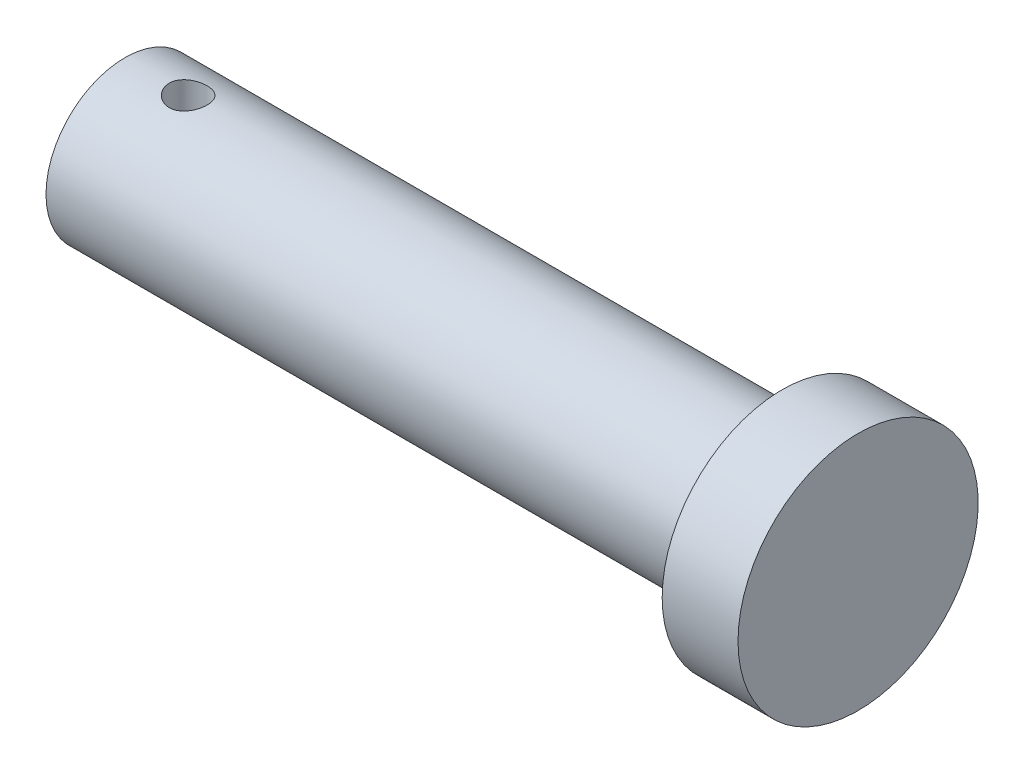
ISO-10303-21;
HEADER;
FILE_DESCRIPTION(('STEP AP214'),'2;1');
FILE_NAME('part.step','',(''),(''),'','','');
FILE_SCHEMA(('AUTOMOTIVE_DESIGN { 1 0 10303 214 1 1 1 1 }'));
ENDSEC;
DATA;
#1=APPLICATION_CONTEXT('core data for automotive mechanical design processes');
#2=APPLICATION_PROTOCOL_DEFINITION('international standard','automotive_design',2000,#1);
#3=PRODUCT_CONTEXT('',#1,'mechanical');
#4=PRODUCT('Part','Part','',(#3));
#5=PRODUCT_RELATED_PRODUCT_CATEGORY('part','',(#4));
#6=PRODUCT_DEFINITION_FORMATION('','',#4);
#7=PRODUCT_DEFINITION_CONTEXT('part definition',#1,'design');
#8=PRODUCT_DEFINITION('design','',#6,#7);
#9=PRODUCT_DEFINITION_SHAPE('','',#8);
#10=(LENGTH_UNIT() NAMED_UNIT(*) SI_UNIT(.MILLI.,.METRE.));
#11=(NAMED_UNIT(*) PLANE_ANGLE_UNIT() SI_UNIT($,.RADIAN.));
#12=(NAMED_UNIT(*) SI_UNIT($,.STERADIAN.) SOLID_ANGLE_UNIT());
#13=UNCERTAINTY_MEASURE_WITH_UNIT(LENGTH_MEASURE(1.E-05),#10,'distance_accuracy_value','');
#14=(GEOMETRIC_REPRESENTATION_CONTEXT(3) GLOBAL_UNCERTAINTY_ASSIGNED_CONTEXT((#13)) GLOBAL_UNIT_ASSIGNED_CONTEXT((#10,
#11,#12)) REPRESENTATION_CONTEXT('',''));
#15=CARTESIAN_POINT('',(0.,0.,0.));
#16=DIRECTION('',(0.,0.,1.));
#17=DIRECTION('',(1.,0.,0.));
#18=AXIS2_PLACEMENT_3D('',#15,#16,#17);
#19=CARTESIAN_POINT('',(0.,0.,0.));
#20=DIRECTION('',(-1.,0.,0.));
#21=DIRECTION('',(0.,0.,1.));
#22=AXIS2_PLACEMENT_3D('',#19,#20,#21);
#23=PLANE('',#22);
#24=CARTESIAN_POINT('',(0.,0.,0.));
#25=DIRECTION('',(-1.,0.,0.));
#26=DIRECTION('',(0.,0.,1.));
#27=AXIS2_PLACEMENT_3D('',#24,#25,#26);
#28=CIRCLE('',#27,12.5);
#29=CARTESIAN_POINT('',(0.,0.,12.5));
#30=VERTEX_POINT('',#29);
#31=EDGE_CURVE('E10',#30,#30,#28,.T.);
#32=ORIENTED_EDGE('',*,*,#31,.T.);
#33=EDGE_LOOP('',(#32));
#34=FACE_BOUND('',#33,.T.);
#35=ADVANCED_FACE('F40',(#34),#23,.T.);
#36=CARTESIAN_POINT('',(-210.,0.,0.));
#37=DIRECTION('',(-1.,0.,0.));
#38=DIRECTION('',(0.,0.,1.));
#39=AXIS2_PLACEMENT_3D('',#36,#37,#38);
#40=CYLINDRICAL_SURFACE('',#39,12.5);
#41=CARTESIAN_POINT('',(10.,-12.1346610995116,3.));
#42=CARTESIAN_POINT('',(9.83411368605636,-12.1346643709057,2.999994926396));
#43=CARTESIAN_POINT('',(9.66816969817756,-12.1380998279897,2.9861940157555));
#44=CARTESIAN_POINT('',(9.34103164728038,-12.1514386999622,2.93143372377318));
#45=CARTESIAN_POINT('',(9.17984063651202,-12.1613461803941,2.89045727127241));
#46=CARTESIAN_POINT('',(8.86698770459709,-12.1864438536979,2.78273587845348));
#47=CARTESIAN_POINT('',(8.71531436580599,-12.2016275682829,2.71602252749926));
#48=CARTESIAN_POINT('',(8.42530045634281,-12.2355589227548,2.55881551789466));
#49=CARTESIAN_POINT('',(8.28696017633045,-12.2543066403104,2.46832134098417));
#50=CARTESIAN_POINT('',(8.02473118505982,-12.2936793084446,2.26416092165145));
#51=CARTESIAN_POINT('',(7.90115284401048,-12.3143323081787,2.15010136587795));
#52=CARTESIAN_POINT('',(7.67468460556583,-12.3549444196641,1.90289576315871));
#53=CARTESIAN_POINT('',(7.57179652880738,-12.3749034702238,1.7697480383165));
#54=CARTESIAN_POINT('',(7.38837356729399,-12.4121875957975,1.48603435008244));
#55=CARTESIAN_POINT('',(7.30814147645071,-12.429475709008,1.33526735140698));
#56=CARTESIAN_POINT('',(7.17427346268216,-12.4591511096292,1.0219036434405));
#57=CARTESIAN_POINT('',(7.12063393185467,-12.471539061815,0.859308542342425));
#58=CARTESIAN_POINT('',(7.04246184561351,-12.4898200905274,0.530137152798909));
#59=CARTESIAN_POINT('',(7.01740278579178,-12.4958305032045,0.363692527540998));
#60=CARTESIAN_POINT('',(6.99545248030836,-12.5010873481438,0.0288605739758578));
#61=CARTESIAN_POINT('',(6.99855738407585,-12.5003347050497,-0.13952648561831));
#62=CARTESIAN_POINT('',(7.03246370078499,-12.4922383642801,-0.469819197188796));
#63=CARTESIAN_POINT('',(7.06269708416856,-12.4850298487431,-0.631786969117105));
#64=CARTESIAN_POINT('',(7.14909173796286,-12.4649879597451,-0.948279915829272));
#65=CARTESIAN_POINT('',(7.20525432510285,-12.4521543006312,-1.10280471220598));
#66=CARTESIAN_POINT('',(7.34238683274778,-12.4220937673228,-1.40154850796015));
#67=CARTESIAN_POINT('',(7.42356325576841,-12.4048305309055,-1.54566890739798));
#68=CARTESIAN_POINT('',(7.60826343366629,-12.3677903650575,-1.8184437481507));
#69=CARTESIAN_POINT('',(7.71179080077328,-12.3480130295253,-1.94709568430374));
#70=CARTESIAN_POINT('',(7.9413154010846,-12.307523454591,-2.18866676072893));
#71=CARTESIAN_POINT('',(8.06780936616896,-12.2868002024656,-2.30111257110785));
#72=CARTESIAN_POINT('',(8.33807563615842,-12.247210122564,-2.50329554889259));
#73=CARTESIAN_POINT('',(8.48184862390316,-12.2283433682075,-2.59303181841777));
#74=CARTESIAN_POINT('',(8.78346525626311,-12.1945661246798,-2.74751986313759));
#75=CARTESIAN_POINT('',(8.94136505107637,-12.1796724534131,-2.81216594132899));
#76=CARTESIAN_POINT('',(9.26623312347684,-12.155748323081,-2.91385324316721));
#77=CARTESIAN_POINT('',(9.43319962468333,-12.1467167199581,-2.95089985341172));
#78=CARTESIAN_POINT('',(9.76709338006787,-12.1357772660229,-2.99556850234642));
#79=CARTESIAN_POINT('',(9.93392207251082,-12.1337008786289,-3.00388683328911));
#80=CARTESIAN_POINT('',(10.2665831940748,-12.1364495609797,-2.99276203410493));
#81=CARTESIAN_POINT('',(10.4324157058037,-12.1412740503119,-2.97332123871795));
#82=CARTESIAN_POINT('',(10.7558459172609,-12.1571201522343,-2.90783852027801));
#83=CARTESIAN_POINT('',(10.9135291759169,-12.1680489760353,-2.86219461484814));
#84=CARTESIAN_POINT('',(11.2190078206671,-12.1947857126682,-2.74603914988784));
#85=CARTESIAN_POINT('',(11.3668021054363,-12.2105941678427,-2.6755248260303));
#86=CARTESIAN_POINT('',(11.651278752204,-12.2456689266469,-2.51014743676234));
#87=CARTESIAN_POINT('',(11.787709374006,-12.2649930224287,-2.41486385815303));
#88=CARTESIAN_POINT('',(12.0429007338939,-12.3047764880024,-2.2031905161038));
#89=CARTESIAN_POINT('',(12.1616588009855,-12.3252360287629,-2.08679756812263));
#90=CARTESIAN_POINT('',(12.3809150096092,-12.3655511140332,-1.8330286051264));
#91=CARTESIAN_POINT('',(12.4809337559897,-12.3853821651221,-1.69523379949056));
#92=CARTESIAN_POINT('',(12.656408463085,-12.4217193399952,-1.4043976180672));
#93=CARTESIAN_POINT('',(12.7318656724447,-12.438225632785,-1.25135701785302));
#94=CARTESIAN_POINT('',(12.855447477275,-12.4659520953338,-0.935406182533391));
#95=CARTESIAN_POINT('',(12.9037623205216,-12.4772089625634,-0.772573732033519));
#96=CARTESIAN_POINT('',(12.9722678203969,-12.4933282808784,-0.440797516621207));
#97=CARTESIAN_POINT('',(12.9924634527555,-12.4981918632553,-0.271854838350954));
#98=CARTESIAN_POINT('',(13.003895867787,-12.5009346170348,0.0628273325379095));
#99=CARTESIAN_POINT('',(12.9958427559416,-12.4989850590467,0.228541548592052));
#100=CARTESIAN_POINT('',(12.9526200369824,-12.4886960978661,0.556181588106274));
#101=CARTESIAN_POINT('',(12.9174511235913,-12.4803568581455,0.718107508375787));
#102=CARTESIAN_POINT('',(12.8213631748843,-12.4582475403262,1.03289533638029));
#103=CARTESIAN_POINT('',(12.7605634305592,-12.4445026408745,1.18579554017999));
#104=CARTESIAN_POINT('',(12.6150497558514,-12.4130357959962,1.47930912419136));
#105=CARTESIAN_POINT('',(12.5303330262537,-12.3953133850962,1.61992106367531));
#106=CARTESIAN_POINT('',(12.3371745257231,-12.3573152907204,1.88826701153781));
#107=CARTESIAN_POINT('',(12.2282449292564,-12.3369914041701,2.01564306622629));
#108=CARTESIAN_POINT('',(11.9907123894103,-12.2963112747441,2.25054951565269));
#109=CARTESIAN_POINT('',(11.8621045592637,-12.2759550250775,2.35807496614236));
#110=CARTESIAN_POINT('',(11.5862606058399,-12.2371275634283,2.5519948518568));
#111=CARTESIAN_POINT('',(11.438747379493,-12.2186938455572,2.63800316633774));
#112=CARTESIAN_POINT('',(11.1309381534945,-12.1862909651906,2.78387070894252));
#113=CARTESIAN_POINT('',(10.9706520843289,-12.1723183758181,2.84375002144869));
#114=CARTESIAN_POINT('',(10.6754071464859,-12.1527391085338,2.92614436386637));
#115=CARTESIAN_POINT('',(10.5419291717888,-12.1460087939348,2.95378236710749));
#116=CARTESIAN_POINT('',(10.2723136259292,-12.1369686046644,2.99071161192546));
#117=CARTESIAN_POINT('',(10.136176245577,-12.1346584140208,3.00000416492674));
#118=CARTESIAN_POINT('',(10.,-12.1346610995116,3.));
#119=B_SPLINE_CURVE_WITH_KNOTS('',3,(#41,#42,#43,#44,#45,#46,#47,#48,#49,#50,#51,#52,#53,#54,
#55,#56,#57,#58,#59,#60,#61,#62,#63,#64,#65,#66,#67,#68,#69,#70,#71,#72,#73,#74,#75,#76,#77,#78,
#79,#80,#81,#82,#83,#84,#85,#86,#87,#88,#89,#90,#91,#92,#93,#94,#95,#96,#97,#98,#99,#100,#101,
#102,#103,#104,#105,#106,#107,#108,#109,#110,#111,#112,#113,#114,#115,#116,#117,#118),
.UNSPECIFIED.,.T.,.F.,(4,2,2,2,2,2,2,2,2,2,2,2,2,2,2,2,2,2,2,2,2,2,2,2,2,2,2,2,2,2,2,2,2,2,2,2,
2,2,4),(0.,0.497159212189434,0.9946310265389,1.49149417875255,1.98836816009861,2.49432418194046,
3.00032470584734,3.51279830766303,4.02520236141813,4.52800628486068,5.03074146609936,
5.52318961529223,6.01566277459448,6.51231571921414,7.00904899016388,7.51819168467209,
8.02735450631453,8.53863957226521,9.04982482437228,9.5485299599376,10.047193153326,
10.5384749824062,11.0298114342859,11.5301065260645,12.0304771548043,12.5422844123508,
13.0540656468818,13.5622134292335,14.0702712827588,14.5656502933719,15.0610166307768,
15.5541024543049,16.047246011943,16.5514085771014,17.0556965465884,17.56847227941,
18.0808531634825,18.4890008491296,18.8971193572843),.UNSPECIFIED.);
#120=CARTESIAN_POINT('',(10.,-12.1346610995116,3.));
#121=VERTEX_POINT('',#120);
#122=EDGE_CURVE('E37',#121,#121,#119,.T.);
#123=ORIENTED_EDGE('',*,*,#122,.F.);
#124=EDGE_LOOP('',(#123));
#125=FACE_BOUND('',#124,.T.);
#126=CARTESIAN_POINT('',(10.,12.1346610995116,3.));
#127=CARTESIAN_POINT('',(10.1658863139436,12.1346643709057,2.999994926396));
#128=CARTESIAN_POINT('',(10.3318303018224,12.1380998279897,2.9861940157555));
#129=CARTESIAN_POINT('',(10.6589683527196,12.1514386999622,2.93143372377318));
#130=CARTESIAN_POINT('',(10.820159363488,12.1613461803941,2.89045727127241));
#131=CARTESIAN_POINT('',(11.1330122954029,12.1864438536979,2.78273587845348));
#132=CARTESIAN_POINT('',(11.284685634194,12.2016275682829,2.71602252749926));
#133=CARTESIAN_POINT('',(11.5746995436572,12.2355589227548,2.55881551789466));
#134=CARTESIAN_POINT('',(11.7130398236696,12.2543066403104,2.46832134098417));
#135=CARTESIAN_POINT('',(11.9752688149402,12.2936793084446,2.26416092165145));
#136=CARTESIAN_POINT('',(12.0988471559895,12.3143323081787,2.15010136587795));
#137=CARTESIAN_POINT('',(12.3253153944342,12.3549444196641,1.90289576315871));
#138=CARTESIAN_POINT('',(12.4282034711926,12.3749034702238,1.76974803831651));
#139=CARTESIAN_POINT('',(12.611626432706,12.4121875957975,1.48603435008245));
#140=CARTESIAN_POINT('',(12.6918585235493,12.429475709008,1.33526735140698));
#141=CARTESIAN_POINT('',(12.8257265373178,12.4591511096292,1.0219036434405));
#142=CARTESIAN_POINT('',(12.8793660681453,12.471539061815,0.859308542342424));
#143=CARTESIAN_POINT('',(12.9575381543865,12.4898200905274,0.530137152798909));
#144=CARTESIAN_POINT('',(12.9825972142082,12.4958305032045,0.363692527540998));
#145=CARTESIAN_POINT('',(13.0045475196916,12.5010873481438,0.0288605739758581));
#146=CARTESIAN_POINT('',(13.0014426159242,12.5003347050497,-0.139526485618309));
#147=CARTESIAN_POINT('',(12.967536299215,12.4922383642801,-0.469819197188796));
#148=CARTESIAN_POINT('',(12.9373029158314,12.4850298487431,-0.631786969117106));
#149=CARTESIAN_POINT('',(12.8509082620371,12.4649879597451,-0.948279915829272));
#150=CARTESIAN_POINT('',(12.7947456748972,12.4521543006312,-1.10280471220598));
#151=CARTESIAN_POINT('',(12.6576131672522,12.4220937673228,-1.40154850796015));
#152=CARTESIAN_POINT('',(12.5764367442316,12.4048305309055,-1.54566890739797));
#153=CARTESIAN_POINT('',(12.3917365663337,12.3677903650575,-1.81844374815069));
#154=CARTESIAN_POINT('',(12.2882091992267,12.3480130295253,-1.94709568430373));
#155=CARTESIAN_POINT('',(12.0586845989154,12.307523454591,-2.18866676072893));
#156=CARTESIAN_POINT('',(11.932190633831,12.2868002024656,-2.30111257110785));
#157=CARTESIAN_POINT('',(11.6619243638416,12.247210122564,-2.50329554889259));
#158=CARTESIAN_POINT('',(11.5181513760968,12.2283433682075,-2.59303181841776));
#159=CARTESIAN_POINT('',(11.2165347437369,12.1945661246798,-2.74751986313759));
#160=CARTESIAN_POINT('',(11.0586349489236,12.1796724534131,-2.81216594132899));
#161=CARTESIAN_POINT('',(10.7337668765232,12.155748323081,-2.91385324316721));
#162=CARTESIAN_POINT('',(10.5668003753167,12.1467167199581,-2.95089985341171));
#163=CARTESIAN_POINT('',(10.2329066199321,12.1357772660229,-2.99556850234642));
#164=CARTESIAN_POINT('',(10.0660779274892,12.1337008786289,-3.00388683328911));
#165=CARTESIAN_POINT('',(9.7334168059252,12.1364495609797,-2.99276203410493));
#166=CARTESIAN_POINT('',(9.56758429419628,12.1412740503119,-2.97332123871795));
#167=CARTESIAN_POINT('',(9.24415408273907,12.1571201522343,-2.90783852027802));
#168=CARTESIAN_POINT('',(9.08647082408308,12.1680489760353,-2.86219461484814));
#169=CARTESIAN_POINT('',(8.78099217933294,12.1947857126682,-2.74603914988784));
#170=CARTESIAN_POINT('',(8.6331978945637,12.2105941678427,-2.67552482603031));
#171=CARTESIAN_POINT('',(8.34872124779605,12.2456689266469,-2.51014743676235));
#172=CARTESIAN_POINT('',(8.21229062599396,12.2649930224287,-2.41486385815303));
#173=CARTESIAN_POINT('',(7.95709926610609,12.3047764880024,-2.20319051610381));
#174=CARTESIAN_POINT('',(7.83834119901455,12.3252360287629,-2.08679756812263));
#175=CARTESIAN_POINT('',(7.61908499039075,12.3655511140332,-1.8330286051264));
#176=CARTESIAN_POINT('',(7.51906624401033,12.3853821651221,-1.69523379949056));
#177=CARTESIAN_POINT('',(7.34359153691497,12.4217193399952,-1.40439761806721));
#178=CARTESIAN_POINT('',(7.26813432755534,12.438225632785,-1.25135701785302));
#179=CARTESIAN_POINT('',(7.14455252272497,12.4659520953338,-0.935406182533393));
#180=CARTESIAN_POINT('',(7.09623767947837,12.4772089625634,-0.77257373203352));
#181=CARTESIAN_POINT('',(7.02773217960313,12.4933282808784,-0.440797516621208));
#182=CARTESIAN_POINT('',(7.00753654724451,12.4981918632553,-0.271854838350955));
#183=CARTESIAN_POINT('',(6.99610413221297,12.5009346170348,0.0628273325379084));
#184=CARTESIAN_POINT('',(7.0041572440584,12.4989850590467,0.228541548592051));
#185=CARTESIAN_POINT('',(7.04737996301755,12.4886960978661,0.556181588106273));
#186=CARTESIAN_POINT('',(7.08254887640871,12.4803568581455,0.718107508375786));
#187=CARTESIAN_POINT('',(7.1786368251157,12.4582475403262,1.03289533638029));
#188=CARTESIAN_POINT('',(7.23943656944082,12.4445026408745,1.18579554017999));
#189=CARTESIAN_POINT('',(7.3849502441486,12.4130357959962,1.47930912419136));
#190=CARTESIAN_POINT('',(7.46966697374628,12.3953133850962,1.61992106367531));
#191=CARTESIAN_POINT('',(7.66282547427691,12.3573152907204,1.88826701153781));
#192=CARTESIAN_POINT('',(7.77175507074358,12.3369914041701,2.01564306622629));
#193=CARTESIAN_POINT('',(8.00928761058973,12.2963112747441,2.25054951565269));
#194=CARTESIAN_POINT('',(8.13789544073631,12.2759550250775,2.35807496614236));
#195=CARTESIAN_POINT('',(8.41373939416014,12.2371275634283,2.5519948518568));
#196=CARTESIAN_POINT('',(8.561252620507,12.2186938455572,2.63800316633774));
#197=CARTESIAN_POINT('',(8.86906184650554,12.1862909651906,2.78387070894252));
#198=CARTESIAN_POINT('',(9.02934791567107,12.1723183758181,2.84375002144869));
#199=CARTESIAN_POINT('',(9.32459285351408,12.1527391085338,2.92614436386637));
#200=CARTESIAN_POINT('',(9.4580708282112,12.1460087939348,2.95378236710749));
#201=CARTESIAN_POINT('',(9.7276863740708,12.1369686046644,2.99071161192546));
#202=CARTESIAN_POINT('',(9.86382375442303,12.1346584140208,3.00000416492674));
#203=CARTESIAN_POINT('',(10.,12.1346610995116,3.));
#204=B_SPLINE_CURVE_WITH_KNOTS('',3,(#126,#127,#128,#129,#130,#131,#132,#133,#134,#135,#136,
#137,#138,#139,#140,#141,#142,#143,#144,#145,#146,#147,#148,#149,#150,#151,#152,#153,#154,#155,
#156,#157,#158,#159,#160,#161,#162,#163,#164,#165,#166,#167,#168,#169,#170,#171,#172,#173,#174,
#175,#176,#177,#178,#179,#180,#181,#182,#183,#184,#185,#186,#187,#188,#189,#190,#191,#192,#193,
#194,#195,#196,#197,#198,#199,#200,#201,#202,#203),.UNSPECIFIED.,.T.,.F.,(4,2,2,2,2,2,2,2,2,2,2,
2,2,2,2,2,2,2,2,2,2,2,2,2,2,2,2,2,2,2,2,2,2,2,2,2,2,2,4),(0.,0.497159212189434,0.9946310265389,
1.49149417875255,1.98836816009861,2.49432418194046,3.00032470584734,3.51279830766303,
4.02520236141814,4.52800628486068,5.03074146609936,5.52318961529223,6.01566277459448,
6.51231571921414,7.00904899016388,7.51819168467208,8.02735450631452,8.53863957226521,
9.04982482437228,9.54852995993759,10.047193153326,10.5384749824062,11.0298114342859,
11.5301065260645,12.0304771548043,12.5422844123508,13.0540656468818,13.5622134292334,
14.0702712827588,14.5656502933719,15.0610166307768,15.5541024543049,16.047246011943,
16.5514085771014,17.0556965465884,17.56847227941,18.0808531634825,18.4890008491296,
18.8971193572843),.UNSPECIFIED.);
#205=CARTESIAN_POINT('',(10.,12.1346610995116,3.));
#206=VERTEX_POINT('',#205);
#207=EDGE_CURVE('E57',#206,#206,#204,.T.);
#208=ORIENTED_EDGE('',*,*,#207,.F.);
#209=EDGE_LOOP('',(#208));
#210=FACE_BOUND('',#209,.T.);
#211=CARTESIAN_POINT('',(104.,0.,0.));
#212=DIRECTION('',(-1.,0.,0.));
#213=DIRECTION('',(0.,0.,1.));
#214=AXIS2_PLACEMENT_3D('',#211,#212,#213);
#215=CIRCLE('',#214,12.5);
#216=CARTESIAN_POINT('',(104.,0.,12.5));
#217=VERTEX_POINT('',#216);
#218=EDGE_CURVE('E48',#217,#217,#215,.T.);
#219=ORIENTED_EDGE('',*,*,#218,.T.);
#220=EDGE_LOOP('',(#219));
#221=FACE_BOUND('',#220,.T.);
#222=ORIENTED_EDGE('',*,*,#31,.F.);
#223=EDGE_LOOP('',(#222));
#224=FACE_BOUND('',#223,.T.);
#225=ADVANCED_FACE('F61',(#125,#210,#221,#224),#40,.T.);
#226=CARTESIAN_POINT('',(104.,-12.5,0.));
#227=DIRECTION('',(-1.,0.,0.));
#228=DIRECTION('',(0.,0.,1.));
#229=AXIS2_PLACEMENT_3D('',#226,#227,#228);
#230=PLANE('',#229);
#231=CARTESIAN_POINT('',(104.,0.,0.));
#232=DIRECTION('',(-1.,0.,0.));
#233=DIRECTION('',(0.,0.,1.));
#234=AXIS2_PLACEMENT_3D('',#231,#232,#233);
#235=CIRCLE('',#234,19.);
#236=CARTESIAN_POINT('',(104.,0.,19.));
#237=VERTEX_POINT('',#236);
#238=EDGE_CURVE('E52',#237,#237,#235,.T.);
#239=ORIENTED_EDGE('',*,*,#238,.T.);
#240=EDGE_LOOP('',(#239));
#241=FACE_BOUND('',#240,.T.);
#242=ORIENTED_EDGE('',*,*,#218,.F.);
#243=EDGE_LOOP('',(#242));
#244=FACE_BOUND('',#243,.T.);
#245=ADVANCED_FACE('F76',(#241,#244),#230,.T.);
#246=CARTESIAN_POINT('',(-210.,0.,0.));
#247=DIRECTION('',(-1.,0.,0.));
#248=DIRECTION('',(0.,0.,1.));
#249=AXIS2_PLACEMENT_3D('',#246,#247,#248);
#250=CYLINDRICAL_SURFACE('',#249,19.);
#251=CARTESIAN_POINT('',(116.,0.,0.));
#252=DIRECTION('',(-1.,0.,0.));
#253=DIRECTION('',(0.,0.,1.));
#254=AXIS2_PLACEMENT_3D('',#251,#252,#253);
#255=CIRCLE('',#254,19.);
#256=CARTESIAN_POINT('',(116.,0.,19.));
#257=VERTEX_POINT('',#256);
#258=EDGE_CURVE('E127',#257,#257,#255,.T.);
#259=ORIENTED_EDGE('',*,*,#258,.T.);
#260=EDGE_LOOP('',(#259));
#261=FACE_BOUND('',#260,.T.);
#262=ORIENTED_EDGE('',*,*,#238,.F.);
#263=EDGE_LOOP('',(#262));
#264=FACE_BOUND('',#263,.T.);
#265=ADVANCED_FACE('F71',(#261,#264),#250,.T.);
#266=CARTESIAN_POINT('',(116.,0.,0.));
#267=DIRECTION('',(1.,0.,0.));
#268=DIRECTION('',(0.,0.,-1.));
#269=AXIS2_PLACEMENT_3D('',#266,#267,#268);
#270=PLANE('',#269);
#271=ORIENTED_EDGE('',*,*,#258,.F.);
#272=EDGE_LOOP('',(#271));
#273=FACE_BOUND('',#272,.T.);
#274=ADVANCED_FACE('F70',(#273),#270,.T.);
#275=CARTESIAN_POINT('',(10.,-19.,0.));
#276=DIRECTION('',(0.,1.,0.));
#277=DIRECTION('',(0.,0.,1.));
#278=AXIS2_PLACEMENT_3D('',#275,#276,#277);
#279=CYLINDRICAL_SURFACE('',#278,3.);
#280=ORIENTED_EDGE('',*,*,#122,.T.);
#281=EDGE_LOOP('',(#280));
#282=FACE_BOUND('',#281,.T.);
#283=ORIENTED_EDGE('',*,*,#207,.T.);
#284=EDGE_LOOP('',(#283));
#285=FACE_BOUND('',#284,.T.);
#286=ADVANCED_FACE('F63',(#282,#285),#279,.F.);
#287=CLOSED_SHELL('',(#35,#225,#245,#265,#274,#286));
#288=MANIFOLD_SOLID_BREP('B2',#287);
#289=ADVANCED_BREP_SHAPE_REPRESENTATION('',(#18,#288),#14);
#290=SHAPE_DEFINITION_REPRESENTATION(#9,#289);
ENDSEC;
END-ISO-10303-21;
